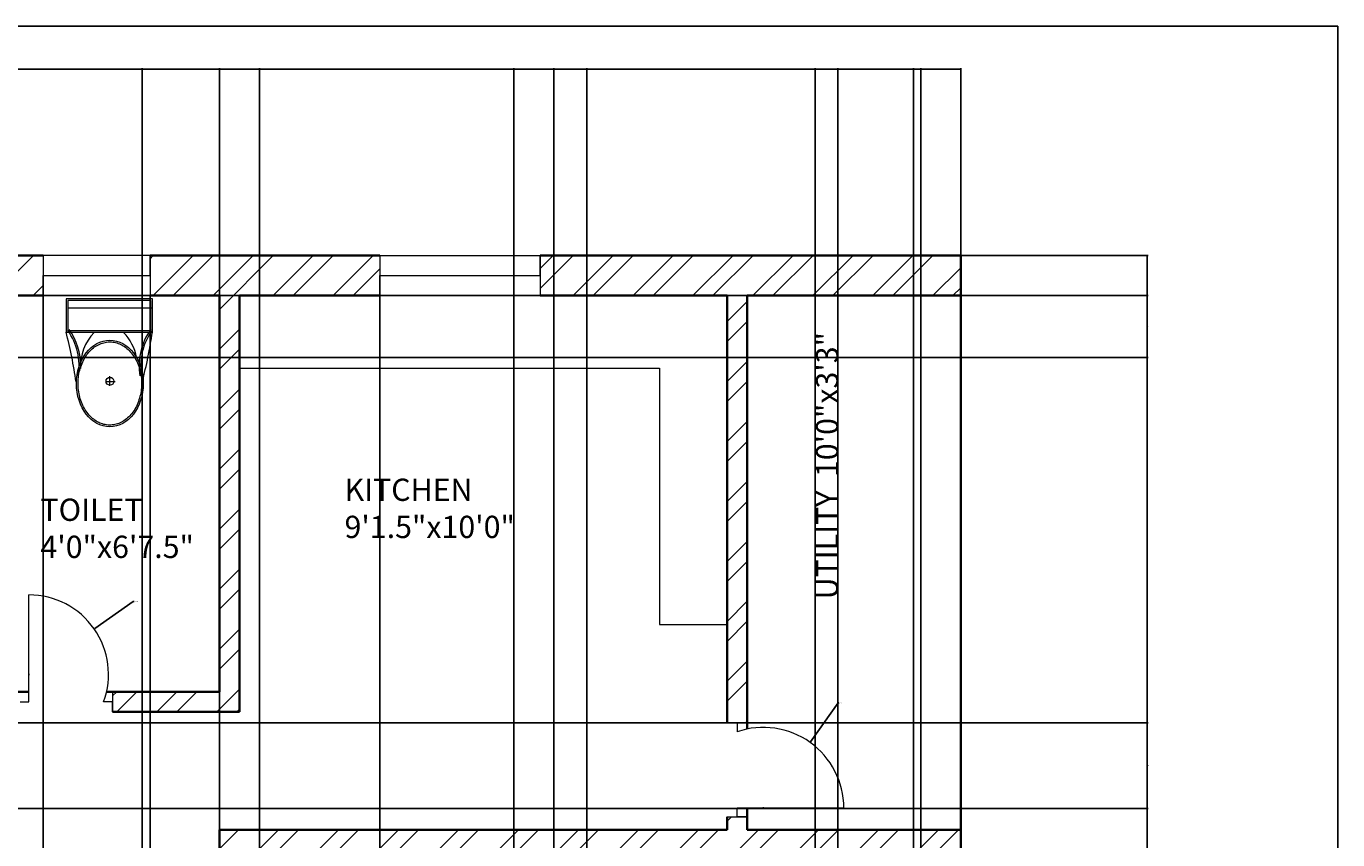
# Model space of a CAD drawing. Units: inches. Extents: x 1748 to 2382, y 1346 to 2284.
# Tile 26 of 26: x 2088 to 2382, y 2102 to 2284. Entities that reach past the tile are written whole.
import ezdxf

# ---------------------------------------------------------------- set-up
doc = ezdxf.new("R2010")
doc.units = ezdxf.units.IN
for name, color, linetype, lineweight in [('A-ANNO-DIMS', 2, 'Continuous', 18), ('A-ANNO-TTLB', 7, 'Continuous', 25), ('A-AREA-IDEN', 7, 'Continuous', 18), ('A-DOOR', 21, 'Continuous', 18), ('A-FLOR-CASE', 32, 'Continuous', 18), ('A-FLOR-FIXT', 7, 'Continuous', 18), ('A-GLAZ', 191, 'Continuous', 18), ('A-WALL', 7, 'Continuous', 35), ('A-WALL-PATT', 9, 'Continuous', 13)]:
    doc.layers.add(name, color=color, linetype=linetype, lineweight=lineweight)
doc.styles.get("Standard").update_dxf_attribs({"font": 'arial.ttf'})
doc.dimstyles.get("Standard").update_dxf_attribs({"dimtxt": 0.18, "dimasz": 0.18, "dimexe": 0.18, "dimexo": 0.0625, "dimgap": 0.09, "dimtad": 0, "dimtih": 1, "dimtoh": 1, "dimdec": 4, "dimzin": 0, "dimdsep": 46, "dimtxsty": 'Standard', "dimcen": 0.09, "dimadec": 0, "dimazin": 0, "dimtfac": 1, "dimtdec": 4, "dimtofl": 0, "dimtmove": 0, "dimatfit": 3, "dimfxl": 1, "dimtolj": 1, "dimtzin": 0, "dimarcsym": 0})

# ---------------------------------------------------------------- blocks, each defined once
blk = doc.blocks.new('A$C31115884')
for p, q in [((283.1, 497.7), (223.4, 497.7)), ((257.5, 466.4), (257.5, 523.2)), ((0, 200), (0, 0)), ((520, 200), (0, 200)), ((10, 190), (10, 10)), ((510, 190), (10, 190)), ((510, 10), (510, 190)), ((520, 0), (520, 200)), ((510, 54.5), (0, 54.5)), ((10, 10), (510, 10)), ((0, 0), (520, 0))]:
    blk.add_line(p, q)
blk.add_circle((255.6, 496.4), 23.6)
for centre, radius, start, end in [((2777.7, -204.6), 2807, 165.4549, 171.71327), ((3237, 905), 2807, 188.28673, 194.5451), ((-294.5, 403.3), 364.7, 324.20913, 9.34987), ((-294.5, 403.3), 374.7, 324.20913, 9.34987), ((139.5, 406.2), 293.5, 315.84364, 2.65635), ((805.8, 403.3), 374.7, 179.20365, 215.79087), ((805.8, 403.3), 364.7, 170.65013, 215.79087), ((383.6, 406.2), 293.5, 190.27735, 224.15636)]:
    blk.add_arc(centre, radius, start, end)
blk.add_ellipse((256.2, 509.9), major_axis=(0, -260.7), ratio=0.772727)
blk.add_open_spline([(256.2, 259.2), (263.1, 259.2), (270, 259.7), (287.8, 262.3), (298.7, 265.1), (319.9, 273.1), (330.2, 278.4), (350.1, 291.1), (359.7, 298.7), (377.7, 315.9), (386.2, 325.5), (401.7, 346.6), (408.8, 358.1), (421.3, 382.5), (426.8, 395.5), (435.9, 422.4), (439.5, 436.4), (444.8, 465.1), (446.5, 479.7), (447.9, 509.2), (447.6, 524), (445, 553.3), (442.7, 567.8), (436.3, 596), (432.1, 609.7), (421.9, 636), (416, 648.6), (402.5, 672.1), (395, 683), (378.6, 703), (369.8, 712.1), (351.1, 728), (341.3, 734.8), (320.9, 746.2), (310.4, 750.7), (288.9, 757.3), (278, 759.4), (256, 761), (245, 760.6), (223.1, 757.2), (212.3, 754.3), (191.1, 746.1), (180.8, 740.7), (160.9, 727.8), (151.4, 720.1), (133.5, 702.7), (125.1, 693), (109.6, 671.7), (102.6, 660.2), (90.2, 635.7), (84.9, 622.7), (76, 595.6), (72.4, 581.6), (67.2, 552.9), (65.6, 538.2), (64.4, 508.8), (64.8, 494), (67.5, 464.7), (69.9, 450.2), (76.6, 422), (80.8, 408.3), (91.1, 382.2), (97.2, 369.7), (110.8, 346.3), (118.4, 335.4), (134.8, 315.6), (143.7, 306.7), (162.4, 290.9), (172.3, 284.2), (192.8, 273), (203.3, 268.6), (224.8, 262.2), (235.8, 260.2), (249.9, 259.3), (253, 259.2), (256.2, 259.2)], degree=3, knots=[0, 0, 0, 0, 0.110105, 0.110105, 0.285049, 0.285049, 0.459994, 0.459994, 0.634938, 0.634938, 0.809882, 0.809882, 0.984827, 0.984827, 1.159771, 1.159771, 1.334715, 1.334715, 1.50966, 1.50966, 1.684604, 1.684604, 1.859549, 1.859549, 2.034493, 2.034493, 2.209437, 2.209437, 2.384382, 2.384382, 2.559326, 2.559326, 2.73427, 2.73427, 2.909215, 2.909215, 3.084159, 3.084159, 3.259103, 3.259103, 3.434048, 3.434048, 3.608992, 3.608992, 3.783936, 3.783936, 3.958881, 3.958881, 4.133825, 4.133825, 4.30877, 4.30877, 4.483714, 4.483714, 4.658658, 4.658658, 4.833603, 4.833603, 5.008547, 5.008547, 5.183491, 5.183491, 5.358436, 5.358436, 5.53338, 5.53338, 5.708324, 5.708324, 5.883269, 5.883269, 6.058213, 6.058213, 6.233158, 6.233158, 6.283185, 6.283185, 6.283185, 6.283185])
blk = doc.blocks.new('WIN-36-DEEP')
for p, q in [((0, 9), (0, 0)), ((0, 9), (36, 9)), ((36, 4.5), (36, 9)), ((36, 9), (36, 0)), ((0, 0), (0, 4.5)), ((0, 4.5), (36, 4.5)), ((36, 0), (0, 0))]:
    blk.add_line(p, q)
blk = doc.blocks.new('*D34')
at = {"layer": 'A-ANNO-DIMS', "color": 0, "lineweight": -2, "transparency": 16777216}
for p, q in [((1821.96, 2232.91), (1821.96, 2274.93)), ((1822.14, 2274.75), (2059.31, 2274.75)), ((2297.28, 2274.75), (2060.11, 2274.75)), ((2297.46, 2232.91), (2297.46, 2274.93))]:
    blk.add_line(p, q, dxfattribs=at)
at = {"layer": 'A-ANNO-DIMS', "color": 0, "transparency": 16777216}
for points in [[(1822.14, 2274.78), (1822.14, 2274.72), (1821.96, 2274.75)], [(2297.28, 2274.78), (2297.28, 2274.72), (2297.46, 2274.75)]]:
    blk.add_solid(points, dxfattribs=at)
at = {"layer": 'Defpoints', "color": 0, "transparency": 16777216}
for p in [(2297.46, 2274.75), (1821.96, 2232.85), (2297.46, 2232.85)]:
    blk.add_point(p, dxfattribs=at)
at = {"layer": 'A-ANNO-DIMS', "color": 0, "transparency": 16777216, "insert": (2059.71, 2274.75), "char_height": 0.18, "attachment_point": 5}
blk.add_mtext('\\A1;475.5', dxfattribs=at)
blk = doc.blocks.new('*D35')
at = {"layer": 'A-ANNO-DIMS', "color": 0, "lineweight": -2, "transparency": 16777216}
for p, q in [((2297.52, 2232.85), (2339.54, 2232.85)), ((2339.36, 2232.67), (2339.36, 1850.53)), ((2339.36, 1468.03), (2339.36, 1850.17)), ((2297.52, 1467.85), (2339.54, 1467.85))]:
    blk.add_line(p, q, dxfattribs=at)
at = {"layer": 'A-ANNO-DIMS', "color": 0, "transparency": 16777216}
for points in [[(2339.33, 2232.67), (2339.39, 2232.67), (2339.36, 2232.85)], [(2339.33, 1468.03), (2339.39, 1468.03), (2339.36, 1467.85)]]:
    blk.add_solid(points, dxfattribs=at)
at = {"layer": 'Defpoints', "color": 0, "transparency": 16777216}
for p in [(2297.46, 2232.85), (2339.36, 2232.85), (2297.46, 1467.85)]:
    blk.add_point(p, dxfattribs=at)
at = {"layer": 'A-ANNO-DIMS', "color": 0, "transparency": 16777216, "insert": (2339.36, 1850.35), "char_height": 0.18, "attachment_point": 5}
blk.add_mtext('\\A1;765', dxfattribs=at)
blk = doc.blocks.new('*D38')
at = {"layer": 'A-ANNO-DIMS', "color": 0, "lineweight": -2, "transparency": 16777216}
for p, q in [((2113.63, 1859.41), (2113.63, 2274.93)), ((2113.81, 2274.75), (2121.84, 2274.75)), ((2130.78, 2274.75), (2122.75, 2274.75)), ((2130.96, 1859.41), (2130.96, 2274.93))]:
    blk.add_line(p, q, dxfattribs=at)
at = {"layer": 'A-ANNO-DIMS', "color": 0, "transparency": 16777216}
for points in [[(2113.81, 2274.78), (2113.81, 2274.72), (2113.63, 2274.75)], [(2130.78, 2274.78), (2130.78, 2274.72), (2130.96, 2274.75)]]:
    blk.add_solid(points, dxfattribs=at)
at = {"layer": 'Defpoints', "color": 0, "transparency": 16777216}
for p in [(2130.96, 2274.75), (2113.63, 1859.35), (2130.96, 1859.35)]:
    blk.add_point(p, dxfattribs=at)
at = {"layer": 'A-ANNO-DIMS', "color": 0, "transparency": 16777216, "insert": (2122.29, 2274.75), "char_height": 0.18, "attachment_point": 5}
blk.add_mtext('\\A1;17.334', dxfattribs=at)
blk = doc.blocks.new('*D39')
at = {"layer": 'A-ANNO-DIMS', "color": 0, "lineweight": -2, "transparency": 16777216}
for p, q in [((2139.96, 1734.91), (2139.96, 2274.93)), ((2140.14, 2274.75), (2168.14, 2274.75)), ((2196.89, 2274.75), (2168.89, 2274.75)), ((2197.07, 1734.91), (2197.07, 2274.93))]:
    blk.add_line(p, q, dxfattribs=at)
at = {"layer": 'A-ANNO-DIMS', "color": 0, "transparency": 16777216}
for points in [[(2140.14, 2274.78), (2140.14, 2274.72), (2139.96, 2274.75)], [(2196.89, 2274.78), (2196.89, 2274.72), (2197.07, 2274.75)]]:
    blk.add_solid(points, dxfattribs=at)
at = {"layer": 'Defpoints', "color": 0, "transparency": 16777216}
for p in [(2197.07, 2274.75), (2139.96, 1734.85), (2197.07, 1734.85)]:
    blk.add_point(p, dxfattribs=at)
at = {"layer": 'A-ANNO-DIMS', "color": 0, "transparency": 16777216, "insert": (2168.52, 2274.75), "char_height": 0.18, "attachment_point": 5}
blk.add_mtext('\\A1;57.11', dxfattribs=at)
blk = doc.blocks.new('*D40')
at = {"layer": 'A-ANNO-DIMS', "color": 0, "lineweight": -2, "transparency": 16777216}
for p, q in [((2206.07, 1734.91), (2206.07, 2274.93)), ((2206.25, 2274.75), (2246.87, 2274.75)), ((2288.28, 2274.75), (2247.66, 2274.75)), ((2288.46, 1734.91), (2288.46, 2274.93))]:
    blk.add_line(p, q, dxfattribs=at)
at = {"layer": 'A-ANNO-DIMS', "color": 0, "transparency": 16777216}
for points in [[(2206.25, 2274.78), (2206.25, 2274.72), (2206.07, 2274.75)], [(2288.28, 2274.78), (2288.28, 2274.72), (2288.46, 2274.75)]]:
    blk.add_solid(points, dxfattribs=at)
at = {"layer": 'Defpoints', "color": 0, "transparency": 16777216}
for p in [(2288.46, 2274.75), (2206.07, 1734.85), (2288.46, 1734.85)]:
    blk.add_point(p, dxfattribs=at)
at = {"layer": 'A-ANNO-DIMS', "color": 0, "transparency": 16777216, "insert": (2247.27, 2274.75), "char_height": 0.18, "attachment_point": 5}
blk.add_mtext('\\A1;82.39', dxfattribs=at)
blk = doc.blocks.new('*D52')
at = {"layer": 'A-ANNO-DIMS', "color": 0, "lineweight": -2, "transparency": 16777216}
for p, q in [((2064.07, 2223.79), (2064.07, 1360.47)), ((2091.4, 2223.79), (2091.4, 1360.47)), ((2064.25, 1360.65), (2077.34, 1360.65)), ((2091.22, 1360.65), (2078.13, 1360.65))]:
    blk.add_line(p, q, dxfattribs=at)
at = {"layer": 'A-ANNO-DIMS', "color": 0, "transparency": 16777216}
for points in [[(2064.25, 1360.68), (2064.25, 1360.62), (2064.07, 1360.65)], [(2091.22, 1360.68), (2091.22, 1360.62), (2091.4, 1360.65)]]:
    blk.add_solid(points, dxfattribs=at)
at = {"layer": 'Defpoints', "color": 0, "transparency": 16777216}
for p in [(2064.07, 2223.85), (2091.4, 2223.85), (2091.4, 1360.65)]:
    blk.add_point(p, dxfattribs=at)
at = {"layer": 'A-ANNO-DIMS', "color": 0, "transparency": 16777216, "insert": (2077.73, 1360.65), "char_height": 0.18, "attachment_point": 5}
blk.add_mtext('\\A1;27.33', dxfattribs=at)
blk = doc.blocks.new('*D53')
at = {"layer": 'A-ANNO-DIMS', "color": 0, "lineweight": -2, "transparency": 16777216}
for p, q in [((2115.4, 2223.79), (2115.4, 1360.47)), ((2167.02, 2223.79), (2167.02, 1360.47)), ((2115.58, 1360.65), (2140.81, 1360.65)), ((2166.84, 1360.65), (2141.6, 1360.65))]:
    blk.add_line(p, q, dxfattribs=at)
at = {"layer": 'A-ANNO-DIMS', "color": 0, "transparency": 16777216}
for points in [[(2115.58, 1360.68), (2115.58, 1360.62), (2115.4, 1360.65)], [(2166.84, 1360.68), (2166.84, 1360.62), (2167.02, 1360.65)]]:
    blk.add_solid(points, dxfattribs=at)
at = {"layer": 'Defpoints', "color": 0, "transparency": 16777216}
for p in [(2115.4, 2223.85), (2167.02, 2223.85), (2167.02, 1360.65)]:
    blk.add_point(p, dxfattribs=at)
at = {"layer": 'A-ANNO-DIMS', "color": 0, "transparency": 16777216, "insert": (2141.21, 1360.65), "char_height": 0.18, "attachment_point": 5}
blk.add_mtext('\\A1;51.62', dxfattribs=at)
blk = doc.blocks.new('*D58')
at = {"layer": 'A-ANNO-DIMS', "color": 0, "lineweight": -2, "transparency": 16777216}
for p, q in [((2269.84, 2064.55), (2269.84, 2274.93)), ((2270.02, 2274.75), (2277.89, 2274.75)), ((2286.67, 2274.75), (2278.8, 2274.75)), ((2286.85, 2064.18), (2286.85, 2274.93))]:
    blk.add_line(p, q, dxfattribs=at)
at = {"layer": 'A-ANNO-DIMS', "color": 0, "transparency": 16777216}
for points in [[(2270.02, 2274.78), (2270.02, 2274.72), (2269.84, 2274.75)], [(2286.67, 2274.78), (2286.67, 2274.72), (2286.85, 2274.75)]]:
    blk.add_solid(points, dxfattribs=at)
at = {"layer": 'Defpoints', "color": 0, "transparency": 16777216}
for p in [(2286.85, 2274.75), (2269.84, 2064.49), (2286.85, 2064.11)]:
    blk.add_point(p, dxfattribs=at)
at = {"layer": 'A-ANNO-DIMS', "color": 0, "transparency": 16777216, "insert": (2278.34, 2274.75), "char_height": 0.18, "attachment_point": 5}
blk.add_mtext('\\A1;17.006', dxfattribs=at)
blk = doc.blocks.new('*D62')
at = {"layer": 'A-ANNO-DIMS', "color": 0, "lineweight": -2, "transparency": 16777216}
for p, q in [((2264.74, 2063.41), (2264.74, 2274.93)), ((2264.92, 2274.75), (2266.9, 2274.75)), ((2269.66, 2274.75), (2267.68, 2274.75)), ((2269.84, 2064.55), (2269.84, 2274.93))]:
    blk.add_line(p, q, dxfattribs=at)
at = {"layer": 'A-ANNO-DIMS', "color": 0, "transparency": 16777216}
for points in [[(2264.92, 2274.78), (2264.92, 2274.72), (2264.74, 2274.75)], [(2269.66, 2274.78), (2269.66, 2274.72), (2269.84, 2274.75)]]:
    blk.add_solid(points, dxfattribs=at)
at = {"layer": 'Defpoints', "color": 0, "transparency": 16777216}
for p in [(2269.84, 2274.75), (2264.74, 2063.35), (2269.84, 2064.49)]:
    blk.add_point(p, dxfattribs=at)
at = {"layer": 'A-ANNO-DIMS', "color": 0, "transparency": 16777216, "insert": (2267.29, 2274.75), "char_height": 0.18, "attachment_point": 5}
blk.add_mtext('\\A1;5.102', dxfattribs=at)
blk = doc.blocks.new('*D68')
at = {"layer": 'A-ANNO-DIMS', "color": 0, "lineweight": -2, "transparency": 16777216}
for p, q in [((1865.52, 2223.85), (2339.54, 2223.85)), ((2339.36, 2223.67), (2339.36, 2217.07)), ((2339.36, 2210.1), (2339.36, 2216.7)), ((1865.52, 2209.92), (2339.54, 2209.92))]:
    blk.add_line(p, q, dxfattribs=at)
at = {"layer": 'A-ANNO-DIMS', "color": 0, "transparency": 16777216}
for points in [[(2339.33, 2223.67), (2339.39, 2223.67), (2339.36, 2223.85)], [(2339.33, 2210.1), (2339.39, 2210.1), (2339.36, 2209.92)]]:
    blk.add_solid(points, dxfattribs=at)
at = {"layer": 'Defpoints', "color": 0, "transparency": 16777216}
for p in [(1865.46, 2223.85), (2339.36, 2223.85), (1865.46, 2209.92)]:
    blk.add_point(p, dxfattribs=at)
at = {"layer": 'A-ANNO-DIMS', "color": 0, "transparency": 16777216, "insert": (2339.36, 2216.88), "char_height": 0.18, "attachment_point": 5}
blk.add_mtext('\\A1;13.93', dxfattribs=at)
blk = doc.blocks.new('*D73')
at = {"layer": 'A-ANNO-DIMS', "color": 0, "lineweight": -2, "transparency": 16777216}
for p, q in [((2139.96, 1979.41), (2139.96, 2274.93)), ((2140.14, 2274.75), (2176.39, 2274.75)), ((2213.28, 2274.75), (2177.03, 2274.75)), ((2213.46, 1979.41), (2213.46, 2274.93))]:
    blk.add_line(p, q, dxfattribs=at)
at = {"layer": 'A-ANNO-DIMS', "color": 0, "transparency": 16777216}
for points in [[(2140.14, 2274.78), (2140.14, 2274.72), (2139.96, 2274.75)], [(2213.28, 2274.78), (2213.28, 2274.72), (2213.46, 2274.75)]]:
    blk.add_solid(points, dxfattribs=at)
at = {"layer": 'Defpoints', "color": 0, "transparency": 16777216}
for p in [(2213.46, 2274.75), (2139.96, 1979.35), (2213.46, 1979.35)]:
    blk.add_point(p, dxfattribs=at)
at = {"layer": 'A-ANNO-DIMS', "color": 0, "transparency": 16777216, "insert": (2176.71, 2274.75), "char_height": 0.18, "attachment_point": 5}
blk.add_mtext('\\A1;73.5', dxfattribs=at)
blk = doc.blocks.new('*D77')
at = {"layer": 'A-ANNO-DIMS', "color": 0, "lineweight": -2, "transparency": 16777216}
for p, q in [((1870.02, 2127.89), (2339.54, 2127.89)), ((2339.36, 2127.71), (2339.36, 2118.43)), ((2339.36, 2108.79), (2339.36, 2118.07)), ((1870.02, 2108.61), (2339.54, 2108.61))]:
    blk.add_line(p, q, dxfattribs=at)
at = {"layer": 'A-ANNO-DIMS', "color": 0, "transparency": 16777216}
for points in [[(2339.33, 2127.71), (2339.39, 2127.71), (2339.36, 2127.89)], [(2339.33, 2108.79), (2339.39, 2108.79), (2339.36, 2108.61)]]:
    blk.add_solid(points, dxfattribs=at)
at = {"layer": 'Defpoints', "color": 0, "transparency": 16777216}
for p in [(1869.96, 2127.89), (2339.36, 2127.89), (1869.96, 2108.61)]:
    blk.add_point(p, dxfattribs=at)
at = {"layer": 'A-ANNO-DIMS', "color": 0, "transparency": 16777216, "insert": (2339.36, 2118.25), "char_height": 0.18, "attachment_point": 5}
blk.add_mtext('\\A1;19.288', dxfattribs=at)
blk = doc.blocks.new('*D90')
at = {"layer": 'A-ANNO-DIMS', "color": 0, "lineweight": -2, "transparency": 16777216}
for p, q in [((2269.92, 2132.33), (2263.72, 2123.63)), ((2270.1, 2132.33), (2269.92, 2132.33)), ((2253.02, 2108.75), (2253.2, 2108.75)), ((2253.11, 2108.66), (2253.11, 2108.84))]:
    blk.add_line(p, q, dxfattribs=at)
at = {"layer": 'A-ANNO-DIMS', "color": 0, "transparency": 16777216}
blk.add_solid([(2263.7, 2123.65), (2263.75, 2123.61), (2263.62, 2123.49)], dxfattribs=at)
at = {"layer": 'Defpoints', "color": 0, "transparency": 16777216}
for p in [(2263.62, 2123.49), (2253.11, 2108.75)]:
    blk.add_point(p, dxfattribs=at)
at = {"layer": 'A-ANNO-DIMS', "color": 0, "transparency": 16777216, "insert": (2270.65, 2132.33), "char_height": 0.18, "attachment_point": 5}
blk.add_mtext('\\A1;R18.096', dxfattribs=at)
blk = doc.blocks.new('*D91')
at = {"layer": 'A-ANNO-DIMS', "color": 0, "lineweight": -2, "transparency": 16777216}
for p, q in [((2111.61, 2155.11), (2102.98, 2149.07)), ((2111.79, 2155.11), (2111.61, 2155.11)), ((2088.1, 2138.74), (2088.28, 2138.74)), ((2088.19, 2138.65), (2088.19, 2138.83))]:
    blk.add_line(p, q, dxfattribs=at)
at = {"layer": 'A-ANNO-DIMS', "color": 0, "transparency": 16777216}
blk.add_solid([(2102.96, 2149.1), (2102.99, 2149.05), (2102.83, 2148.97)], dxfattribs=at)
at = {"layer": 'Defpoints', "color": 0, "transparency": 16777216}
for p in [(2102.83, 2148.97), (2088.19, 2138.74)]:
    blk.add_point(p, dxfattribs=at)
at = {"layer": 'A-ANNO-DIMS', "color": 0, "transparency": 16777216, "insert": (2112.27, 2155.11), "char_height": 0.18, "attachment_point": 5}
blk.add_mtext('\\A1;R17.86', dxfattribs=at)

msp = doc.modelspace()

# ---------------------------------------------------------------- hatches: boundary and pattern name
at = {"layer": 'A-WALL-PATT'}
h = msp.add_hatch(dxfattribs=at)
h.set_pattern_fill('ANSI32', color=256)
h.paths.add_polyline_path([(1908.4445, 2232.8497), (1821.9607, 2232.8497), (1821.9607, 2223.8497), (1865.4607, 2223.8497), (1865.4607, 2209.9185), (1869.9607, 2209.9185), (1869.9607, 2223.8497), (1908.4445, 2223.8497), (1908.4445, 2228.3497)])
h.paths.add_polyline_path([(2040.0683, 2232.8497), (1968.4445, 2232.8497), (1968.4445, 2223.8497), (2025.9607, 2223.8497), (2025.9607, 2130.3497), (2032.1341, 2130.3497), (2032.1341, 2132.5997), (2032.1341, 2134.8497), (2030.4607, 2134.8497), (2030.4607, 2223.8497), (2040.0683, 2223.8497)])
h.paths.add_polyline_path([(2091.3969, 2232.8497), (2064.0683, 2232.8497), (2064.0683, 2223.8497), (2078.4607, 2223.8497), (2078.4607, 2134.8497), (2051.1563, 2134.8497), (2051.1563, 2130.3497), (2078.4607, 2130.3497), (2078.4607, 2128.6813), (2082.9607, 2128.6813), (2082.9607, 2130.3497), (2086.1879, 2130.3497), (2086.1879, 2132.5997), (2086.1879, 2134.8497), (2082.9607, 2134.8497), (2082.9607, 2223.8497), (2091.3969, 2223.8497), (2091.3969, 2228.3497)])
h.paths.add_polyline_path([(2167.0164, 2232.8497), (2115.3969, 2232.8497), (2115.3969, 2223.8497), (2130.9607, 2223.8497), (2130.9607, 2134.8497), (2106.9607, 2134.8497), (2106.9607, 2130.3497), (2135.4607, 2130.3497), (2135.4607, 2223.8497), (2167.0164, 2223.8497), (2167.0164, 2228.3497)])
h.paths.add_polyline_path([(1869.9607, 2149.9185), (1865.4607, 2149.9185), (1865.4607, 2127.8942), (1869.9607, 2127.8942)])
h.paths.add_polyline_path([(2082.9607, 2104.4871), (2080.7107, 2104.4871), (2078.4607, 2104.4871), (2078.4607, 2103.8497), (1869.9607, 2103.8497), (1869.9607, 2108.6062), (1867.7107, 2108.6062), (1865.4607, 2108.6062), (1865.4607, 2103.8497), (1821.9607, 2103.8497), (1821.9607, 2099.3497), (1865.4607, 2099.3497), (1865.4607, 2094.7509), (1869.9607, 2094.7509), (1869.9607, 2099.3497), (2025.9607, 2099.3497), (2025.9607, 2096.4326), (2030.4607, 2096.4326), (2030.4607, 2099.3497), (2082.9607, 2099.3497)])
h.paths.add_polyline_path([(1928.9457, 1401.1212), (2176.8693, 1401.1212), (2176.8693, 1438.214), (1928.9457, 1438.214)], flags=9)
h.paths.add_polyline_path([(2122.2668, 2048.1927), (2177.9387, 2048.1927), (2177.9387, 2066.85), (2122.2668, 2066.85)], flags=9)
h.paths.add_polyline_path([(2272.688, 2153.8197), (2272.688, 2216.746), (2262.3845, 2216.746), (2262.3845, 2153.8197)], flags=9)
h.paths.add_polyline_path([(2157.2928, 2166.5593), (2196.3822, 2166.5593), (2196.3822, 2185.2167), (2157.2928, 2185.2167)], flags=9)
h.paths.add_polyline_path([(2089.3407, 2162.0698), (2124.3987, 2162.0698), (2124.3987, 2180.7272), (2089.3407, 2180.7272)], flags=9)
h.paths.add_polyline_path([(2037.4521, 2160.0913), (2072.5101, 2160.0913), (2072.5101, 2178.7486), (2037.4521, 2178.7486)], flags=9)
h.paths.add_polyline_path([(1884.7894, 2104.1554), (1923.6297, 2104.1554), (1923.6297, 2122.8127), (1884.7894, 2122.8127)], flags=9)
h.paths.add_polyline_path([(1851.2832, 2142.9749), (1851.2832, 2199.3051), (1840.9796, 2199.3051), (1840.9796, 2142.9749)], flags=9)
h.paths.add_polyline_path([(1844.8763, 2017.2834), (1844.8763, 2073.6136), (1834.5728, 2073.6136), (1834.5728, 2017.2834)], flags=9)
h.paths.add_polyline_path([(1897.1577, 2073.1279), (1935.9981, 2073.1279), (1935.9981, 2091.7853), (1897.1577, 2091.7853)], flags=9)
h.paths.add_polyline_path([(1952.3395, 1802.4231), (2008.0114, 1802.4231), (2008.0114, 1821.0805), (1952.3395, 1821.0805)], flags=9)
h.paths.add_polyline_path([(1978.8184, 1857.6841), (2017.7338, 1857.6841), (2017.7338, 1876.3415), (1978.8184, 1876.3415)], flags=9)
h.paths.add_polyline_path([(1979.6513, 1925.9516), (2008.8089, 1925.9516), (2008.8089, 1944.6089), (1979.6513, 1944.6089)], flags=9)
h.paths.add_polyline_path([(1838.5553, 1860.3527), (1877.3957, 1860.3527), (1877.3957, 1879.01), (1838.5553, 1879.01)], flags=9)
h.paths.add_polyline_path([(1883.9018, 1787.3013), (1883.9018, 1843.6315), (1873.5983, 1843.6315), (1873.5983, 1787.3013)], flags=9)
h.paths.add_polyline_path([(1873.7079, 1509.1938), (1873.7079, 1583.7709), (1863.4044, 1583.7709), (1863.4044, 1509.1938)], flags=9)
h.paths.add_polyline_path([(1916.2259, 1603.3681), (1955.0663, 1603.3681), (1955.0663, 1622.0254), (1916.2259, 1622.0254)], flags=9)
h.paths.add_polyline_path([(1876.3013, 1636.757), (1876.3013, 1693.0871), (1865.9978, 1693.0871), (1865.9978, 1636.757)], flags=9)
h.paths.add_polyline_path([(1921.3138, 1521.8316), (1964.0662, 1521.8316), (1964.0662, 1540.489), (1921.3138, 1540.489)], flags=9)
h.paths.add_polyline_path([(2017.5657, 1497.5078), (2046.7983, 1497.5078), (2046.7983, 1516.1651), (2017.5657, 1516.1651)], flags=9)
h.paths.add_polyline_path([(2066.8661, 1499.3902), (2096.0988, 1499.3902), (2096.0988, 1518.0475), (2066.8661, 1518.0475)], flags=9)
h.paths.add_polyline_path([(2155.4835, 1571.6596), (2198.2358, 1571.6596), (2198.2358, 1590.3169), (2155.4835, 1590.3169)], flags=9)
h.paths.add_polyline_path([(2094.9136, 1664.6812), (2150.5855, 1664.6812), (2150.5855, 1683.3386), (2094.9136, 1683.3386)], flags=9)
h.paths.add_polyline_path([(2257.6902, 1863.1628), (2269.8935, 1863.1628), (2269.8935, 1873.4664), (2257.6902, 1873.4664)], flags=9)
h.paths.add_polyline_path([(2164.0748, 1880.3089), (2189.8694, 1880.3089), (2189.8694, 1890.6124), (2164.0748, 1890.6124)], flags=9)
h.paths.add_polyline_path([(2239.4394, 1931.0585), (2268.8187, 1931.0585), (2268.8187, 1949.7159), (2239.4394, 1949.7159)], flags=9)
h = msp.add_hatch(dxfattribs=at)
h.set_pattern_fill('ANSI32', color=256)
h.paths.add_polyline_path([(2297.4607, 2232.8497), (2203.0164, 2232.8497), (2203.0164, 2223.8497), (2244.9607, 2223.8497), (2244.9607, 2127.8554), (2249.4607, 2127.8554), (2249.4607, 2223.8497), (2297.4607, 2223.8497)])
h.paths.add_polyline_path([(2297.4607, 2103.8497), (2249.4607, 2103.8497), (2249.4607, 2106.7497), (2247.2107, 2106.7497), (2244.9607, 2106.7497), (2244.9607, 2103.8497), (2130.9607, 2103.8497), (2130.9607, 2099.3497), (2288.4607, 2099.3497), (2288.4607, 2077.2008), (2297.4607, 2077.2008)])
h.paths.add_polyline_path([(1928.9457, 1401.1212), (2176.8693, 1401.1212), (2176.8693, 1438.214), (1928.9457, 1438.214)], flags=9)
h.paths.add_polyline_path([(2122.2668, 2048.1927), (2177.9387, 2048.1927), (2177.9387, 2066.85), (2122.2668, 2066.85)], flags=9)
h.paths.add_polyline_path([(2272.688, 2153.8197), (2272.688, 2216.746), (2262.3845, 2216.746), (2262.3845, 2153.8197)], flags=25)
h.paths.add_polyline_path([(2157.2928, 2166.5593), (2196.3822, 2166.5593), (2196.3822, 2185.2167), (2157.2928, 2185.2167)], flags=9)
h.paths.add_polyline_path([(2089.3407, 2162.0698), (2124.3987, 2162.0698), (2124.3987, 2180.7272), (2089.3407, 2180.7272)], flags=9)
h.paths.add_polyline_path([(2037.4521, 2160.0913), (2072.5101, 2160.0913), (2072.5101, 2178.7486), (2037.4521, 2178.7486)], flags=9)
h.paths.add_polyline_path([(1884.7894, 2104.1554), (1923.6297, 2104.1554), (1923.6297, 2122.8127), (1884.7894, 2122.8127)], flags=9)
h.paths.add_polyline_path([(1851.2832, 2142.9749), (1851.2832, 2199.3051), (1840.9796, 2199.3051), (1840.9796, 2142.9749)], flags=9)
h.paths.add_polyline_path([(1844.8763, 2017.2834), (1844.8763, 2073.6136), (1834.5728, 2073.6136), (1834.5728, 2017.2834)], flags=9)
h.paths.add_polyline_path([(1897.1577, 2073.1279), (1935.9981, 2073.1279), (1935.9981, 2091.7853), (1897.1577, 2091.7853)], flags=9)
h.paths.add_polyline_path([(1952.3395, 1802.4231), (2008.0114, 1802.4231), (2008.0114, 1821.0805), (1952.3395, 1821.0805)], flags=9)
h.paths.add_polyline_path([(1978.8184, 1857.6841), (2017.7338, 1857.6841), (2017.7338, 1876.3415), (1978.8184, 1876.3415)], flags=9)
h.paths.add_polyline_path([(1979.6513, 1925.9516), (2008.8089, 1925.9516), (2008.8089, 1944.6089), (1979.6513, 1944.6089)], flags=9)
h.paths.add_polyline_path([(1838.5553, 1860.3527), (1877.3957, 1860.3527), (1877.3957, 1879.01), (1838.5553, 1879.01)], flags=9)
h.paths.add_polyline_path([(1883.9018, 1787.3013), (1883.9018, 1843.6315), (1873.5983, 1843.6315), (1873.5983, 1787.3013)], flags=9)
h.paths.add_polyline_path([(1873.7079, 1509.1938), (1873.7079, 1583.7709), (1863.4044, 1583.7709), (1863.4044, 1509.1938)], flags=9)
h.paths.add_polyline_path([(1916.2259, 1603.3681), (1955.0663, 1603.3681), (1955.0663, 1622.0254), (1916.2259, 1622.0254)], flags=9)
h.paths.add_polyline_path([(1876.3013, 1636.757), (1876.3013, 1693.0871), (1865.9978, 1693.0871), (1865.9978, 1636.757)], flags=9)
h.paths.add_polyline_path([(1921.3138, 1521.8316), (1964.0662, 1521.8316), (1964.0662, 1540.489), (1921.3138, 1540.489)], flags=9)
h.paths.add_polyline_path([(2017.5657, 1497.5078), (2046.7983, 1497.5078), (2046.7983, 1516.1651), (2017.5657, 1516.1651)], flags=9)
h.paths.add_polyline_path([(2066.8661, 1499.3902), (2096.0988, 1499.3902), (2096.0988, 1518.0475), (2066.8661, 1518.0475)], flags=9)
h.paths.add_polyline_path([(2155.4835, 1571.6596), (2198.2358, 1571.6596), (2198.2358, 1590.3169), (2155.4835, 1590.3169)], flags=9)
h.paths.add_polyline_path([(2094.9136, 1664.6812), (2150.5855, 1664.6812), (2150.5855, 1683.3386), (2094.9136, 1683.3386)], flags=9)
h.paths.add_polyline_path([(2257.6902, 1863.1628), (2269.8935, 1863.1628), (2269.8935, 1873.4664), (2257.6902, 1873.4664)], flags=9)
h.paths.add_polyline_path([(2164.0748, 1880.3089), (2189.8694, 1880.3089), (2189.8694, 1890.6124), (2164.0748, 1890.6124)], flags=9)
h.paths.add_polyline_path([(2239.4394, 1931.0585), (2268.8187, 1931.0585), (2268.8187, 1949.7159), (2239.4394, 1949.7159)], flags=9)
h = msp.add_hatch(dxfattribs=at)
h.set_pattern_fill('ANSI32', color=256)
h.paths.add_polyline_path([(1919.6777, 1476.8497), (1900.6426, 1476.8497), (1900.6426, 1522.0826), (1898.3926, 1522.0826), (1896.1426, 1522.0826), (1896.1426, 1476.8497), (1857.1426, 1476.8497), (1857.1426, 1467.8497), (1896.1426, 1467.8497), (1919.6777, 1467.8497), (1919.6777, 1472.3497)])
h.paths.add_polyline_path([(2018.7873, 1472.3497), (2018.7873, 1476.8497), (2010.9607, 1476.8497), (2010.9607, 1560.8497), (2034.9607, 1560.8497), (2034.9607, 1565.3497), (2006.4607, 1565.3497), (2006.4607, 1476.8497), (1955.6777, 1476.8497), (1955.6777, 1467.8497), (2018.7873, 1467.8497)])
h.paths.add_polyline_path([(2152.3354, 1472.3497), (2152.3354, 1476.8497), (2115.9607, 1476.8497), (2115.9607, 1565.3497), (2109.2204, 1565.3497), (2109.2204, 1563.0997), (2109.2204, 1560.8497), (2111.4607, 1560.8497), (2111.4607, 1476.8497), (2095.3617, 1476.8497), (2095.3617, 1467.8497), (2152.3354, 1467.8497)])
h.paths.add_polyline_path([(2071.3617, 1476.8497), (2063.4607, 1476.8497), (2063.4607, 1560.8497), (2090.1865, 1560.8497), (2090.1865, 1565.3497), (2063.4607, 1565.3497), (2063.4607, 1572.5485), (2061.2107, 1572.5485), (2058.9607, 1572.5485), (2058.9607, 1565.3497), (2055.6281, 1565.3497), (2055.6281, 1560.8497), (2058.9607, 1560.8497), (2058.9607, 1476.8497), (2042.7873, 1476.8497), (2042.7873, 1467.8497), (2071.3617, 1467.8497), (2071.3617, 1472.3497)])
h.paths.add_polyline_path([(2297.4607, 1506.5652), (2288.4607, 1506.5652), (2288.4607, 1476.8497), (2212.3354, 1476.8497), (2212.3354, 1467.8497), (2297.4607, 1467.8497)])
h.paths.add_polyline_path([(2297.4607, 1645.3038), (2288.4607, 1645.3038), (2288.4607, 1605.8497), (2058.9607, 1605.8497), (2058.9607, 1600.1857), (2061.2107, 1600.1857), (2063.4607, 1600.1857), (2063.4607, 1601.3497), (2288.4607, 1601.3497), (2288.4607, 1566.5652), (2297.4607, 1566.5652)])
h.paths.add_polyline_path([(2010.9607, 1609.0561), (2008.7107, 1609.0561), (2006.4607, 1609.0561), (2006.4607, 1605.8497), (1900.6426, 1605.8497), (1900.6426, 1609.7171), (1898.3926, 1609.7171), (1896.1426, 1609.7171), (1896.1426, 1605.8497), (1857.1426, 1605.8497), (1857.1426, 1601.3497), (1896.1426, 1601.3497), (1896.1426, 1542.5447), (1900.6426, 1542.5447), (1900.6426, 1601.3497), (2010.9607, 1601.3497)])
h.paths.add_polyline_path([(1928.9457, 1401.1212), (2176.8693, 1401.1212), (2176.8693, 1438.214), (1928.9457, 1438.214)], flags=9)
h.paths.add_polyline_path([(2122.2668, 2048.1927), (2177.9387, 2048.1927), (2177.9387, 2066.85), (2122.2668, 2066.85)], flags=9)
h.paths.add_polyline_path([(2272.688, 2153.8197), (2272.688, 2216.746), (2262.3845, 2216.746), (2262.3845, 2153.8197)], flags=9)
h.paths.add_polyline_path([(2157.2928, 2166.5593), (2196.3822, 2166.5593), (2196.3822, 2185.2167), (2157.2928, 2185.2167)], flags=9)
h.paths.add_polyline_path([(2089.3407, 2162.0698), (2124.3987, 2162.0698), (2124.3987, 2180.7272), (2089.3407, 2180.7272)], flags=9)
h.paths.add_polyline_path([(2037.4521, 2160.0913), (2072.5101, 2160.0913), (2072.5101, 2178.7486), (2037.4521, 2178.7486)], flags=9)
h.paths.add_polyline_path([(1884.7894, 2104.1554), (1923.6297, 2104.1554), (1923.6297, 2122.8127), (1884.7894, 2122.8127)], flags=9)
h.paths.add_polyline_path([(1851.2832, 2142.9749), (1851.2832, 2199.3051), (1840.9796, 2199.3051), (1840.9796, 2142.9749)], flags=9)
h.paths.add_polyline_path([(1844.8763, 2017.2834), (1844.8763, 2073.6136), (1834.5728, 2073.6136), (1834.5728, 2017.2834)], flags=9)
h.paths.add_polyline_path([(1897.1577, 2073.1279), (1935.9981, 2073.1279), (1935.9981, 2091.7853), (1897.1577, 2091.7853)], flags=9)
h.paths.add_polyline_path([(1952.3395, 1802.4231), (2008.0114, 1802.4231), (2008.0114, 1821.0805), (1952.3395, 1821.0805)], flags=9)
h.paths.add_polyline_path([(1978.8184, 1857.6841), (2017.7338, 1857.6841), (2017.7338, 1876.3415), (1978.8184, 1876.3415)], flags=9)
h.paths.add_polyline_path([(1979.6513, 1925.9516), (2008.8089, 1925.9516), (2008.8089, 1944.6089), (1979.6513, 1944.6089)], flags=9)
h.paths.add_polyline_path([(1838.5553, 1860.3527), (1877.3957, 1860.3527), (1877.3957, 1879.01), (1838.5553, 1879.01)], flags=9)
h.paths.add_polyline_path([(1883.9018, 1787.3013), (1883.9018, 1843.6315), (1873.5983, 1843.6315), (1873.5983, 1787.3013)], flags=9)
h.paths.add_polyline_path([(1873.7079, 1509.1938), (1873.7079, 1583.7709), (1863.4044, 1583.7709), (1863.4044, 1509.1938)], flags=9)
h.paths.add_polyline_path([(1916.2259, 1603.3681), (1955.0663, 1603.3681), (1955.0663, 1622.0254), (1916.2259, 1622.0254)], flags=9)
h.paths.add_polyline_path([(1876.3013, 1636.757), (1876.3013, 1693.0871), (1865.9978, 1693.0871), (1865.9978, 1636.757)], flags=9)
h.paths.add_polyline_path([(1921.3138, 1521.8316), (1964.0662, 1521.8316), (1964.0662, 1540.489), (1921.3138, 1540.489)], flags=9)
h.paths.add_polyline_path([(2017.5657, 1497.5078), (2046.7983, 1497.5078), (2046.7983, 1516.1651), (2017.5657, 1516.1651)], flags=9)
h.paths.add_polyline_path([(2066.8661, 1499.3902), (2096.0988, 1499.3902), (2096.0988, 1518.0475), (2066.8661, 1518.0475)], flags=9)
h.paths.add_polyline_path([(2155.4835, 1571.6596), (2198.2358, 1571.6596), (2198.2358, 1590.3169), (2155.4835, 1590.3169)], flags=25)
h.paths.add_polyline_path([(2094.9136, 1664.6812), (2150.5855, 1664.6812), (2150.5855, 1683.3386), (2094.9136, 1683.3386)], flags=9)
h.paths.add_polyline_path([(2257.6902, 1863.1628), (2269.8935, 1863.1628), (2269.8935, 1873.4664), (2257.6902, 1873.4664)], flags=9)
h.paths.add_polyline_path([(2164.0748, 1880.3089), (2189.8694, 1880.3089), (2189.8694, 1890.6124), (2164.0748, 1890.6124)], flags=9)
h.paths.add_polyline_path([(2239.4394, 1931.0585), (2268.8187, 1931.0585), (2268.8187, 1949.7159), (2239.4394, 1949.7159)], flags=9)

# ---------------------------------------------------------------- linework, layer by layer
at = {"layer": 'A-ANNO-TTLB'}
msp.add_lwpolyline([(1747.8112, 2284.3704), (2382.1361, 2284.3704), (2382.1361, 1346.4899), (1747.8112, 1346.4899)], close=True, dxfattribs=at)
at = {"layer": 'A-DOOR'}
for p, q in [((2088.1879, 2132.5997), (2088.1879, 2156.5997)), ((2106.9607, 2134.8497), (2106.9607, 2130.3497)), ((2086.1879, 2132.5997), (2088.1879, 2132.5997)), ((2106.9607, 2132.5997), (2104.9607, 2132.5997)), ((2106.9607, 2130.3497), (2106.9607, 2132.5997)), ((2244.9607, 2127.8554), (2249.4607, 2127.8554)), ((2249.4607, 2127.8554), (2247.2107, 2127.8554)), ((2247.2107, 2127.8554), (2247.2107, 2125.8554)), ((2244.9607, 2106.7497), (2249.4607, 2106.7497)), ((2247.2107, 2106.7497), (2247.2107, 2108.7497)), ((2247.2107, 2108.7497), (2271.2107, 2108.7497)), ((2249.4607, 2106.7497), (2247.2107, 2106.7497))]:
    msp.add_line(p, q, dxfattribs=at)
for centre, radius, start, end in [((2088.1879, 2138.7387), 17.8609, 339.896662, 90), ((2253.1147, 2108.7497), 18.096, 360, 109.04209)]:
    msp.add_arc(centre, radius, start, end, dxfattribs=at)
at = {"layer": 'A-FLOR-CASE'}
for p, q in [((2135.4607, 2207.5272), (2229.7677, 2207.5272)), ((2229.7677, 2207.5272), (2229.7677, 2149.9321)), ((2229.7677, 2149.9321), (2244.9607, 2149.9321))]:
    msp.add_line(p, q, dxfattribs=at)
at = {"layer": 'A-GLAZ'}
for p, q in [((2091.3969, 2232.8497), (2091.3969, 2232.8497)), ((2091.3969, 2232.8497), (2091.3969, 2223.8497)), ((2115.3969, 2232.8497), (2091.3969, 2232.8497)), ((2115.3969, 2228.3497), (2115.3969, 2232.8497)), ((2115.3969, 2232.8497), (2115.3969, 2223.8497)), ((2091.3969, 2223.8497), (2091.3969, 2228.3497)), ((2091.3969, 2228.3497), (2115.3969, 2228.3497)), ((2115.3969, 2223.8497), (2091.3969, 2223.8497))]:
    msp.add_line(p, q, dxfattribs=at)
at = {"layer": 'A-WALL'}
for p, q in [((2064.0683, 2232.8497), (2091.3969, 2232.8497)), ((2115.3969, 2232.8497), (2167.0164, 2232.8497)), ((2203.0164, 2232.8497), (2297.4607, 2232.8497)), ((2297.4607, 2232.8497), (2297.4607, 2077.2008)), ((2082.9607, 2223.8497), (2091.3969, 2223.8497)), ((2115.3969, 2223.8497), (2130.9607, 2223.8497)), ((2130.9607, 2223.8497), (2130.9607, 2134.8497)), ((2135.4607, 2223.8497), (2135.4607, 2130.3497)), ((2135.4607, 2223.8497), (2167.0164, 2223.8497)), ((2203.0164, 2223.8497), (2244.9607, 2223.8497)), ((2244.9607, 2223.8497), (2244.9607, 2127.8554)), ((2249.4607, 2223.8497), (2249.4607, 2126.4729)), ((2249.4607, 2223.8497), (2297.4607, 2223.8497)), ((2082.9607, 2134.8497), (2088.1879, 2134.8497)), ((2105.6203, 2134.8497), (2130.9607, 2134.8497)), ((2106.9607, 2130.3497), (2135.4607, 2130.3497)), ((2244.9607, 2106.7497), (2244.9607, 2103.8497)), ((2249.4607, 2108.7497), (2249.4607, 2103.8497)), ((2130.9607, 2103.8497), (2244.9607, 2103.8497)), ((2130.9607, 2099.3497), (2130.9607, 2103.8497)), ((2249.4607, 2103.8497), (2297.4607, 2103.8497))]:
    msp.add_line(p, q, dxfattribs=at)

# ---------------------------------------------------------------- block references
at = {"layer": 'A-FLOR-FIXT', "xscale": 0.0372717239612423, "yscale": 0.0372717239612423, "zscale": 0.0372717239612423, "rotation": 180}
msp.add_blockref('A$C31115884', (2115.8925, 2223.1115), dxfattribs=at)
at = {"layer": 'A-GLAZ'}
msp.add_blockref('WIN-36-DEEP', (2167.0167, 2223.85), dxfattribs=at)

# ---------------------------------------------------------------- texts
at = {"layer": 'A-AREA-IDEN', "insert": (2264.9374, 2155.6188), "char_height": 5, "attachment_point": 1, "rotation": 90}
msp.add_mtext_dynamic_manual_height_columns('UTILITY  10\'0"x3\'3"', width=192.515564, gutter_width=12.5, heights=[0], dxfattribs=at)
at = {"layer": 'A-AREA-IDEN', "char_height": 5, "attachment_point": 1}
for s, width, insert in [('KITCHEN\\P9\'1.5"x10\'0"', 118.259794, (2159.0544, 2182.7286)), ('TOILET\\P4\'0"x6\'7.5"', 87.237183, (2090.7544, 2178.2425))]:
    msp.add_mtext_dynamic_manual_height_columns(s, width=width, gutter_width=12.5, heights=[0], dxfattribs=dict(at, insert=insert))

# ---------------------------------------------------------------- dimensions: what is measured, and where the dimension line sits
at = {"layer": 'A-ANNO-DIMS'}
for base, p1, p2, override, picture, middle in [((2297.4607, 2274.7497), (1821.9607, 2232.8497), (2297.4607, 2232.8497), {"dimdec": 1, "dimlfac": 1, "dimrnd": 0, "dimzin": 0, "dimdsep": 46, "dimlunit": 2}, '*D34', (2059.7107, 2274.7497)), ((2130.9607, 2274.7497), (2113.6268, 1859.3497), (2130.9607, 1859.3497), {"dimdec": 3, "dimlfac": 1, "dimrnd": 0, "dimzin": 0, "dimdsep": 46, "dimlunit": 2}, '*D38', (2122.2937, 2274.7497)), ((2197.0699, 2274.7497), (2139.9607, 1734.8497), (2197.0699, 1734.8497), {"dimdec": 2, "dimlfac": 1, "dimrnd": 0, "dimzin": 0, "dimdsep": 46, "dimlunit": 2}, '*D39', (2168.5153, 2274.7497)), ((2213.4607, 2274.7497), (2139.9607, 1979.3497), (2213.4607, 1979.3497), {"dimdec": 1, "dimlfac": 1, "dimrnd": 0, "dimzin": 0, "dimdsep": 46, "dimlunit": 2}, '*D73', (2176.7107, 2274.7497)), ((2288.4607, 2274.7497), (2206.0699, 1734.8497), (2288.4607, 1734.8497), {"dimdec": 2, "dimlfac": 1, "dimrnd": 0, "dimzin": 0, "dimdsep": 46, "dimlunit": 2}, '*D40', (2247.2653, 2274.7497)), ((2269.8419, 2274.7497), (2264.7402, 2063.352), (2269.8419, 2064.4916), {"dimdec": 3, "dimlfac": 1, "dimrnd": 0, "dimzin": 0, "dimdsep": 46, "dimlunit": 2}, '*D62', (2267.2911, 2274.7497)), ((2286.8477, 2274.7497), (2269.8419, 2064.4916), (2286.8477, 2064.1137), {"dimdec": 3, "dimlfac": 1, "dimrnd": 0, "dimzin": 0, "dimdsep": 46, "dimlunit": 2}, '*D58', (2278.3448, 2274.7497)), ((2091.3969, 1360.6451), (2064.0683, 2223.8497), (2091.3969, 2223.8497), {"dimdec": 2, "dimlfac": 1, "dimrnd": 0, "dimzin": 0, "dimdsep": 46, "dimlunit": 2}, '*D52', (2077.7326, 1360.6451)), ((2167.0164, 1360.6451), (2115.3969, 2223.8497), (2167.0164, 2223.8497), {"dimdec": 2, "dimlfac": 1, "dimrnd": 0, "dimzin": 0, "dimdsep": 46, "dimlunit": 2}, '*D53', (2141.2066, 1360.6451))]:
    dim = msp.add_linear_dim(base=base, p1=p1, p2=p2, dimstyle='Standard', override=override, dxfattribs=at)
    dim.commit()
    dim.dimension.update_dxf_attribs({"geometry": picture, "text_midpoint": middle})
for base, p1, p2, override, picture, middle in [((2339.3607, 2232.8497), (2297.4607, 1467.8497), (2297.4607, 2232.8497), {"dimdec": 0, "dimlfac": 1, "dimrnd": 0, "dimzin": 0, "dimdsep": 46, "dimlunit": 2}, '*D35', (2339.3607, 1850.3497)), ((2339.3607, 2223.8497), (1865.4607, 2209.9185), (1865.4607, 2223.8497), {"dimdec": 2, "dimlfac": 1, "dimrnd": 0, "dimzin": 0, "dimdsep": 46, "dimlunit": 2}, '*D68', (2339.3607, 2216.8841)), ((2339.3607, 2127.8942), (1869.9607, 2108.6062), (1869.9607, 2127.8942), {"dimdec": 3, "dimlfac": 1, "dimrnd": 0, "dimzin": 0, "dimdsep": 46, "dimlunit": 2}, '*D77', (2339.3607, 2118.2502))]:
    dim = msp.add_linear_dim(base=base, p1=p1, p2=p2, angle=90, dimstyle='Standard', override=override, dxfattribs=at)
    dim.commit()
    dim.dimension.update_dxf_attribs({"geometry": picture, "text_midpoint": middle})
for center, mpoint, override, picture, middle in [((2088.1879, 2138.7387), (2102.828, 2148.97), {"dimdec": 2, "dimlfac": 1, "dimrnd": 0, "dimzin": 0, "dimdsep": 46, "dimlunit": 2}, '*D91', (2112.2719, 2155.1088)), ((2253.1147, 2108.7497), (2263.6178, 2123.4857), {"dimdec": 3, "dimlfac": 1, "dimrnd": 0, "dimzin": 0, "dimdsep": 46, "dimlunit": 2}, '*D90', (2270.6493, 2132.3273))]:
    dim = msp.add_radius_dim(center=center, mpoint=mpoint, dimstyle='Standard', override=override, dxfattribs=at)
    dim.commit()
    dim.dimension.update_dxf_attribs({"geometry": picture, "text_midpoint": middle, "dimtype": 164})

doc.saveas('drawing.dxf')
